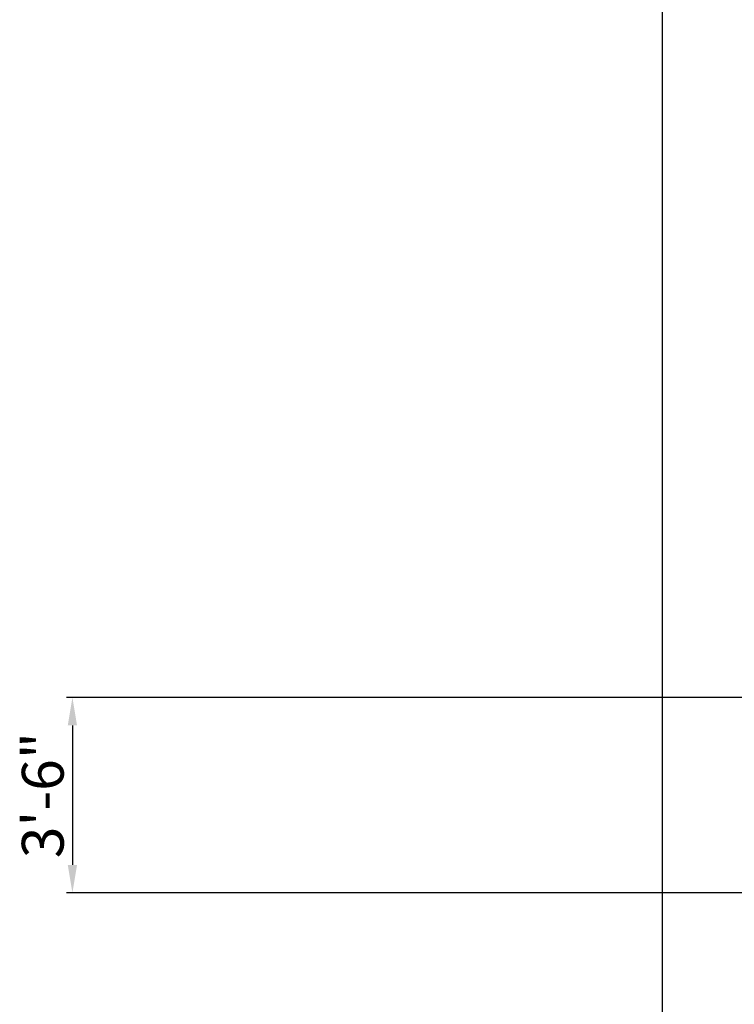
# Model space of a CAD drawing. Units: millimetres. Extents: x 595116 to 630915, y 909473 to 920225.
# Tile 112 of 134: x 629144 to 629298, y 919346 to 919558. Entities that reach past the tile are written whole.
import ezdxf

# ---------------------------------------------------------------- set-up
doc = ezdxf.new("R2010")
doc.units = ezdxf.units.MM
doc.layers.add('Dimension', color=3, linetype='Continuous', lineweight=18)
doc.styles.get("Standard").update_dxf_attribs({"font": 'arial.ttf'})
doc.dimstyles.new('ISO-25', dxfattribs={"dimtxt": 9, "dimasz": 6, "dimexe": 1.25, "dimexo": 0.625, "dimtad": 1, "dimlunit": 4, "dimtxsty": 'Standard', "dimcen": 2.5, "dimadec": 0, "dimazin": 0, "dimtfac": 1, "dimtmove": 0, "dimatfit": 3, "dimfxl": 1, "dimarcsym": 0})

# ---------------------------------------------------------------- blocks, each defined once
blk = doc.blocks.new('*D128')
at = {"layer": 'Defpoints', "color": 0, "transparency": 16777216}
for p in [(629311.54, 920089.43), (629282.4, 919141.93), (629311.54, 919141.93)]:
    blk.add_point(p, dxfattribs=at)
at = {"layer": 'Dimension', "color": 0, "lineweight": -2, "transparency": 16777216}
for p, q in [((629310.92, 920089.43), (629281.15, 920089.43)), ((629282.4, 920083.43), (629282.4, 919147.93)), ((629310.92, 919141.93), (629281.15, 919141.93))]:
    blk.add_line(p, q, dxfattribs=at)
at = {"layer": 'Dimension', "color": 0, "transparency": 16777216}
for points in [[(629281.4, 920083.43), (629283.4, 920083.43), (629282.4, 920089.43)], [(629281.4, 919147.93), (629283.4, 919147.93), (629282.4, 919141.93)]]:
    blk.add_solid(points, dxfattribs=at)
at = {"layer": 'Dimension', "color": 0, "transparency": 16777216, "insert": (629271.16, 919615.68), "char_height": 9, "attachment_point": 5, "rotation": 90}
blk.add_mtext('78\'-11{\\H1x;\\S1/2;}"', dxfattribs=at)
blk = doc.blocks.new('*D217')
at = {"layer": 'Defpoints', "color": 0, "transparency": 16777216}
for p in [(629743.54, 919411.93), (629155.38, 919369.93), (629743.54, 919369.93)]:
    blk.add_point(p, dxfattribs=at)
at = {"layer": 'Dimension', "color": 0, "lineweight": -2, "transparency": 16777216}
for p, q in [((629742.92, 919411.93), (629154.13, 919411.93)), ((629155.38, 919405.93), (629155.38, 919375.93)), ((629742.92, 919369.93), (629154.13, 919369.93))]:
    blk.add_line(p, q, dxfattribs=at)
at = {"layer": 'Dimension', "color": 0, "transparency": 16777216}
for points in [[(629154.38, 919405.93), (629156.38, 919405.93), (629155.38, 919411.93)], [(629154.38, 919375.93), (629156.38, 919375.93), (629155.38, 919369.93)]]:
    blk.add_solid(points, dxfattribs=at)
at = {"layer": 'Dimension', "color": 0, "transparency": 16777216, "insert": (629150.16, 919390.93), "char_height": 9, "attachment_point": 5, "rotation": 90}
blk.add_mtext('3\'-6"', dxfattribs=at)

msp = doc.modelspace()

# ---------------------------------------------------------------- dimensions: what is measured, and where the dimension line sits
at = {"layer": 'Dimension'}
for base, p1, p2, override, picture, middle in [((629282.395, 919141.928), (629311.541, 920089.428), (629311.541, 919141.928), {"dimclrd": 0, "dimclre": 0, "dimclrt": 0}, '*D128', (629271.157, 919615.678)), ((629155.382, 919369.928), (629743.541, 919411.928), (629743.541, 919369.928), {"dimdec": 1, "dimlfac": 1, "dimrnd": 0, "dimzin": 1, "dimdsep": 46, "dimlunit": 4, "dimfrac": 2}, '*D217', (629150.159, 919390.928))]:
    dim = msp.add_linear_dim(base=base, p1=p1, p2=p2, angle=90, dimstyle='ISO-25', override=override, dxfattribs=at)
    dim.commit()
    dim.dimension.update_dxf_attribs({"geometry": picture, "text_midpoint": middle})

doc.saveas('drawing.dxf')
